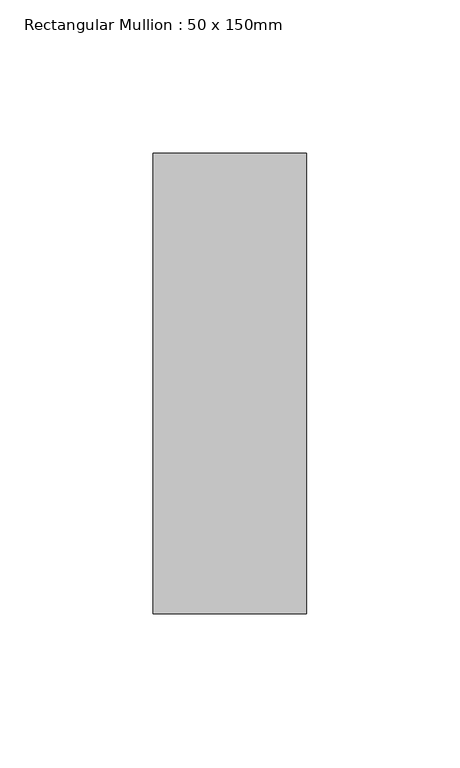
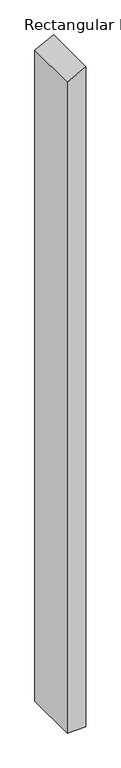
"""IFC4 building model written with IfcOpenShell, lengths in millimetres: member geometry, Rectangular Mullion : 50 x 150mm."""

from ifc_helpers import new_model, si_unit, frame, origin, place, context, project, spatial, polyline, outline, extrude, source, transform, mapped, element, save


def rectangular_mullion_50_x_150mm_9159db86(model_context):
    return source(origin(), model_context, "Body", "SweptSolid", [
        extrude(outline(polyline([(0.0, 0.0), (-26.0283525, -50.0), (-1876.6744496, -50.0), (-1876.6744496, 0.0), (0.0, 0.0)])), frame((0.0, -75.0, 0.0), z_axis=(0.0, 1.0, 0.0), x_axis=(0.0, 0.0, 1.0)), (0.0, 0.0, 1.0), 150.0),
    ])


if __name__ == "__main__":
    model = new_model("IFC4")
    model_context = context("Model", 3, world=origin())
    ifc_project = project(units=[si_unit("LENGTHUNIT", "METRE", prefix="MILLI")], contexts=[model_context])
    site = spatial("IfcSite", under=ifc_project)
    building = spatial("IfcBuilding", under=site)
    placement = place(None, origin())
    rectangular_mullion_50_x_150mm_shape = rectangular_mullion_50_x_150mm_9159db86(model_context)
    element("IfcMember", 1, ObjectType="Rectangular Mullion : 50 x 150mm", at=placement, inside=building, context=model_context, shape_type="MappedRepresentation", body=[
        mapped(rectangular_mullion_50_x_150mm_shape, transform((0.0, 0.0, 0.0), x_axis=(1.0, 0.0, 0.0), y_axis=(0.0, 1.0, 0.0), z_axis=(0.0, 0.0, 1.0))),
    ])
    save(model, "model.ifc")

# Revit data of these elements
# Type "Rectangular Mullion : 50 x 150mm"
#   built-in parameter 1007304 = 0.492126 (stored number, unit not read)
#   built-in parameter 1007301 = 0.082021 (stored number, unit not read)
#   built-in parameter 1007300 = 0.082021 (stored number, unit not read)
# Element 1 (IfcMember, "Rectangular Mullion : 50 x 150mm")
#   Materials on its faces: "Aluminium"
# Materials
#   "Aluminium": class "Metal", colour RGB 247 247 247, transparency 0, Description = "Aluminium 6061", Cost = 0
